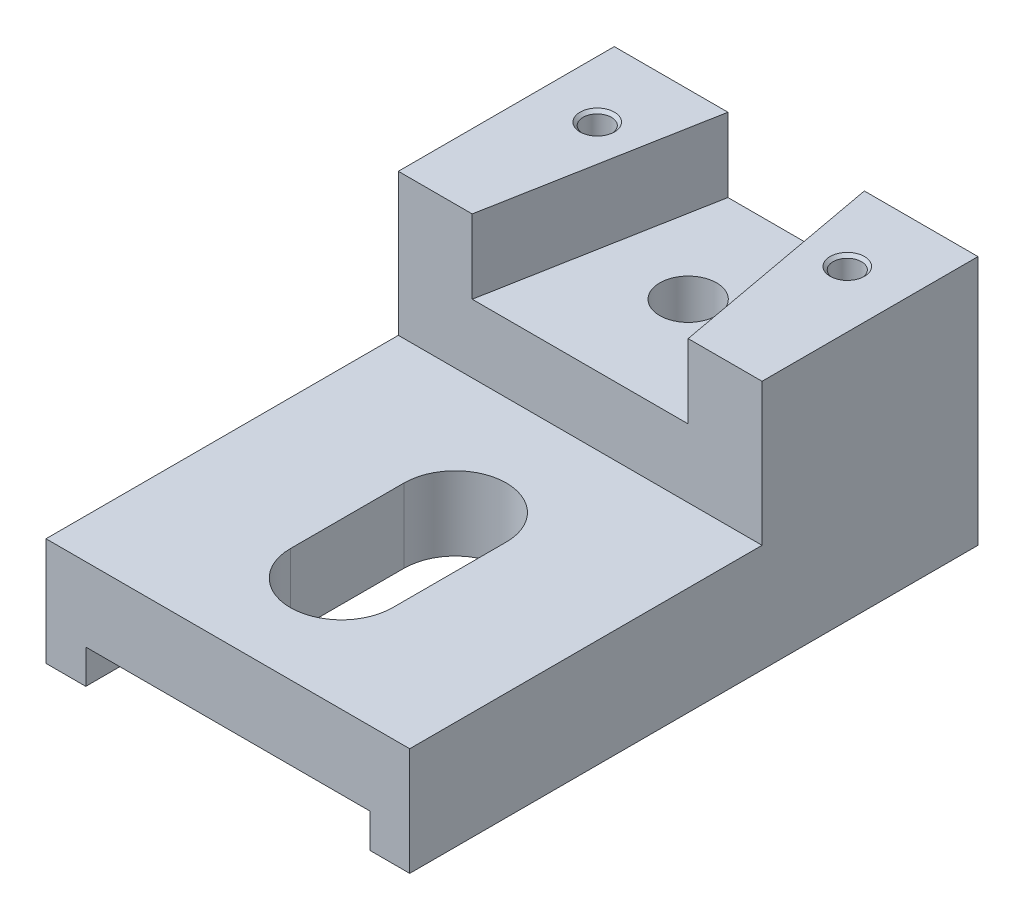
ISO-10303-21;
HEADER;
FILE_DESCRIPTION(('STEP AP214'),'2;1');
FILE_NAME('part.step','',(''),(''),'','','');
FILE_SCHEMA(('AUTOMOTIVE_DESIGN { 1 0 10303 214 1 1 1 1 }'));
ENDSEC;
DATA;
#1=APPLICATION_CONTEXT('core data for automotive mechanical design processes');
#2=APPLICATION_PROTOCOL_DEFINITION('international standard','automotive_design',2000,#1);
#3=PRODUCT_CONTEXT('',#1,'mechanical');
#4=PRODUCT('Part','Part','',(#3));
#5=PRODUCT_RELATED_PRODUCT_CATEGORY('part','',(#4));
#6=PRODUCT_DEFINITION_FORMATION('','',#4);
#7=PRODUCT_DEFINITION_CONTEXT('part definition',#1,'design');
#8=PRODUCT_DEFINITION('design','',#6,#7);
#9=PRODUCT_DEFINITION_SHAPE('','',#8);
#10=(LENGTH_UNIT() NAMED_UNIT(*) SI_UNIT(.MILLI.,.METRE.));
#11=(NAMED_UNIT(*) PLANE_ANGLE_UNIT() SI_UNIT($,.RADIAN.));
#12=(NAMED_UNIT(*) SI_UNIT($,.STERADIAN.) SOLID_ANGLE_UNIT());
#13=UNCERTAINTY_MEASURE_WITH_UNIT(LENGTH_MEASURE(1.E-05),#10,'distance_accuracy_value','');
#14=(GEOMETRIC_REPRESENTATION_CONTEXT(3) GLOBAL_UNCERTAINTY_ASSIGNED_CONTEXT((#13)) GLOBAL_UNIT_ASSIGNED_CONTEXT((#10,
#11,#12)) REPRESENTATION_CONTEXT('',''));
#15=CARTESIAN_POINT('',(0.,0.,0.));
#16=DIRECTION('',(0.,0.,1.));
#17=DIRECTION('',(1.,0.,0.));
#18=AXIS2_PLACEMENT_3D('',#15,#16,#17);
#19=CARTESIAN_POINT('',(-19.,38.,-62.));
#20=DIRECTION('',(-0.983453188589073,0.,-0.181162429476935));
#21=DIRECTION('',(-0.181162429476935,0.,0.983453188589073));
#22=AXIS2_PLACEMENT_3D('',#19,#20,#21);
#23=PLANE('',#22);
#24=DIRECTION('',(-0.181162429476935,0.,0.983453188589073));
#25=VECTOR('',#24,1.);
#26=CARTESIAN_POINT('',(-19.,25.,-62.));
#27=LINE('',#26,#25);
#28=CARTESIAN_POINT('',(-12.,25.,-100.));
#29=VERTEX_POINT('',#28);
#30=CARTESIAN_POINT('',(-19.,25.,-62.));
#31=VERTEX_POINT('',#30);
#32=EDGE_CURVE('E204',#29,#31,#27,.T.);
#33=ORIENTED_EDGE('',*,*,#32,.F.);
#34=DIRECTION('',(0.,-1.,0.));
#35=VECTOR('',#34,1.);
#36=CARTESIAN_POINT('',(-12.,38.,-100.));
#37=LINE('',#36,#35);
#38=CARTESIAN_POINT('',(-12.,38.,-100.));
#39=VERTEX_POINT('',#38);
#40=EDGE_CURVE('E233',#39,#29,#37,.T.);
#41=ORIENTED_EDGE('',*,*,#40,.F.);
#42=DIRECTION('',(0.181162429476935,0.,-0.983453188589073));
#43=VECTOR('',#42,1.);
#44=CARTESIAN_POINT('',(-19.,38.,-62.));
#45=LINE('',#44,#43);
#46=CARTESIAN_POINT('',(-19.,38.,-62.));
#47=VERTEX_POINT('',#46);
#48=EDGE_CURVE('E248',#47,#39,#45,.T.);
#49=ORIENTED_EDGE('',*,*,#48,.F.);
#50=DIRECTION('',(0.,-1.,0.));
#51=VECTOR('',#50,1.);
#52=CARTESIAN_POINT('',(-19.,38.,-62.));
#53=LINE('',#52,#51);
#54=EDGE_CURVE('E261',#47,#31,#53,.T.);
#55=ORIENTED_EDGE('',*,*,#54,.T.);
#56=EDGE_LOOP('',(#33,#41,#49,#55));
#57=FACE_BOUND('',#56,.T.);
#58=ADVANCED_FACE('F43',(#57),#23,.F.);
#59=CARTESIAN_POINT('',(19.,38.,-62.));
#60=DIRECTION('',(0.983453188589073,0.,-0.181162429476935));
#61=DIRECTION('',(-0.181162429476935,0.,-0.983453188589073));
#62=AXIS2_PLACEMENT_3D('',#59,#60,#61);
#63=PLANE('',#62);
#64=DIRECTION('',(-0.181162429476935,0.,-0.983453188589073));
#65=VECTOR('',#64,1.);
#66=CARTESIAN_POINT('',(12.,25.,-100.));
#67=LINE('',#66,#65);
#68=CARTESIAN_POINT('',(19.,25.,-62.));
#69=VERTEX_POINT('',#68);
#70=CARTESIAN_POINT('',(12.,25.,-100.));
#71=VERTEX_POINT('',#70);
#72=EDGE_CURVE('E207',#69,#71,#67,.T.);
#73=ORIENTED_EDGE('',*,*,#72,.F.);
#74=DIRECTION('',(0.,-1.,0.));
#75=VECTOR('',#74,1.);
#76=CARTESIAN_POINT('',(19.,38.,-62.));
#77=LINE('',#76,#75);
#78=CARTESIAN_POINT('',(19.,38.,-62.));
#79=VERTEX_POINT('',#78);
#80=EDGE_CURVE('E249',#79,#69,#77,.T.);
#81=ORIENTED_EDGE('',*,*,#80,.F.);
#82=DIRECTION('',(0.181162429476935,0.,0.983453188589073));
#83=VECTOR('',#82,1.);
#84=CARTESIAN_POINT('',(19.,38.,-62.));
#85=LINE('',#84,#83);
#86=CARTESIAN_POINT('',(12.,38.,-100.));
#87=VERTEX_POINT('',#86);
#88=EDGE_CURVE('E232',#87,#79,#85,.T.);
#89=ORIENTED_EDGE('',*,*,#88,.F.);
#90=DIRECTION('',(0.,-1.,0.));
#91=VECTOR('',#90,1.);
#92=CARTESIAN_POINT('',(12.,38.,-100.));
#93=LINE('',#92,#91);
#94=EDGE_CURVE('E252',#87,#71,#93,.T.);
#95=ORIENTED_EDGE('',*,*,#94,.T.);
#96=EDGE_LOOP('',(#73,#81,#89,#95));
#97=FACE_BOUND('',#96,.T.);
#98=ADVANCED_FACE('F363',(#97),#63,.F.);
#99=CARTESIAN_POINT('',(-25.,0.,-100.));
#100=DIRECTION('',(1.,0.,0.));
#101=DIRECTION('',(0.,0.,-1.));
#102=AXIS2_PLACEMENT_3D('',#99,#100,#101);
#103=PLANE('',#102);
#104=DIRECTION('',(0.,1.,0.));
#105=VECTOR('',#104,1.);
#106=CARTESIAN_POINT('',(-25.,0.,0.));
#107=LINE('',#106,#105);
#108=CARTESIAN_POINT('',(-25.,-6.00000000000001,0.));
#109=VERTEX_POINT('',#108);
#110=CARTESIAN_POINT('',(-25.,0.,0.));
#111=VERTEX_POINT('',#110);
#112=EDGE_CURVE('E254',#109,#111,#107,.T.);
#113=ORIENTED_EDGE('',*,*,#112,.F.);
#114=DIRECTION('',(0.,0.,1.));
#115=VECTOR('',#114,1.);
#116=CARTESIAN_POINT('',(-25.,-6.00000000000001,-100.));
#117=LINE('',#116,#115);
#118=CARTESIAN_POINT('',(-25.,-6.00000000000001,-100.));
#119=VERTEX_POINT('',#118);
#120=EDGE_CURVE('E320',#119,#109,#117,.T.);
#121=ORIENTED_EDGE('',*,*,#120,.F.);
#122=DIRECTION('',(0.,1.,0.));
#123=VECTOR('',#122,1.);
#124=CARTESIAN_POINT('',(-25.,0.,-100.));
#125=LINE('',#124,#123);
#126=CARTESIAN_POINT('',(-25.,0.,-100.));
#127=VERTEX_POINT('',#126);
#128=EDGE_CURVE('E272',#119,#127,#125,.T.);
#129=ORIENTED_EDGE('',*,*,#128,.T.);
#130=DIRECTION('',(0.,0.,1.));
#131=VECTOR('',#130,1.);
#132=CARTESIAN_POINT('',(-25.,0.,-100.));
#133=LINE('',#132,#131);
#134=EDGE_CURVE('E294',#127,#111,#133,.T.);
#135=ORIENTED_EDGE('',*,*,#134,.T.);
#136=EDGE_LOOP('',(#113,#121,#129,#135));
#137=FACE_BOUND('',#136,.T.);
#138=ADVANCED_FACE('F44',(#137),#103,.T.);
#139=CARTESIAN_POINT('',(-25.,-6.00000000000001,-100.));
#140=DIRECTION('',(0.,-1.,0.));
#141=DIRECTION('',(1.,0.,0.));
#142=AXIS2_PLACEMENT_3D('',#139,#140,#141);
#143=PLANE('',#142);
#144=DIRECTION('',(1.,0.,0.));
#145=VECTOR('',#144,1.);
#146=CARTESIAN_POINT('',(-25.,-6.00000000000001,0.));
#147=LINE('',#146,#145);
#148=CARTESIAN_POINT('',(-32.,-6.00000000000001,0.));
#149=VERTEX_POINT('',#148);
#150=EDGE_CURVE('E280',#149,#109,#147,.T.);
#151=ORIENTED_EDGE('',*,*,#150,.F.);
#152=DIRECTION('',(0.,0.,1.));
#153=VECTOR('',#152,1.);
#154=CARTESIAN_POINT('',(-32.,-6.00000000000001,-100.));
#155=LINE('',#154,#153);
#156=CARTESIAN_POINT('',(-32.,-6.00000000000001,-100.));
#157=VERTEX_POINT('',#156);
#158=EDGE_CURVE('E319',#157,#149,#155,.T.);
#159=ORIENTED_EDGE('',*,*,#158,.F.);
#160=DIRECTION('',(1.,0.,0.));
#161=VECTOR('',#160,1.);
#162=CARTESIAN_POINT('',(-25.,-6.00000000000001,-100.));
#163=LINE('',#162,#161);
#164=EDGE_CURVE('E292',#157,#119,#163,.T.);
#165=ORIENTED_EDGE('',*,*,#164,.T.);
#166=ORIENTED_EDGE('',*,*,#120,.T.);
#167=EDGE_LOOP('',(#151,#159,#165,#166));
#168=FACE_BOUND('',#167,.T.);
#169=ADVANCED_FACE('F387',(#168),#143,.T.);
#170=CARTESIAN_POINT('',(-32.,-6.00000000000001,-100.));
#171=DIRECTION('',(-1.,0.,0.));
#172=DIRECTION('',(0.,0.,1.));
#173=AXIS2_PLACEMENT_3D('',#170,#171,#172);
#174=PLANE('',#173);
#175=DIRECTION('',(0.,-1.,0.));
#176=VECTOR('',#175,1.);
#177=CARTESIAN_POINT('',(-32.,-6.00000000000001,0.));
#178=LINE('',#177,#176);
#179=CARTESIAN_POINT('',(-32.,13.,0.));
#180=VERTEX_POINT('',#179);
#181=EDGE_CURVE('E315',#180,#149,#178,.T.);
#182=ORIENTED_EDGE('',*,*,#181,.F.);
#183=DIRECTION('',(0.,0.,1.));
#184=VECTOR('',#183,1.);
#185=CARTESIAN_POINT('',(-32.,13.,-100.));
#186=LINE('',#185,#184);
#187=CARTESIAN_POINT('',(-32.,13.,-62.));
#188=VERTEX_POINT('',#187);
#189=EDGE_CURVE('E325',#188,#180,#186,.T.);
#190=ORIENTED_EDGE('',*,*,#189,.F.);
#191=DIRECTION('',(0.,-1.,0.));
#192=VECTOR('',#191,1.);
#193=CARTESIAN_POINT('',(-32.,38.,-62.));
#194=LINE('',#193,#192);
#195=CARTESIAN_POINT('',(-32.,38.,-62.));
#196=VERTEX_POINT('',#195);
#197=EDGE_CURVE('E256',#196,#188,#194,.T.);
#198=ORIENTED_EDGE('',*,*,#197,.F.);
#199=DIRECTION('',(0.,0.,1.));
#200=VECTOR('',#199,1.);
#201=CARTESIAN_POINT('',(-32.,38.,-100.));
#202=LINE('',#201,#200);
#203=CARTESIAN_POINT('',(-32.,38.,-100.));
#204=VERTEX_POINT('',#203);
#205=EDGE_CURVE('E266',#204,#196,#202,.T.);
#206=ORIENTED_EDGE('',*,*,#205,.F.);
#207=DIRECTION('',(0.,-1.,0.));
#208=VECTOR('',#207,1.);
#209=CARTESIAN_POINT('',(-32.,-6.00000000000001,-100.));
#210=LINE('',#209,#208);
#211=EDGE_CURVE('E286',#204,#157,#210,.T.);
#212=ORIENTED_EDGE('',*,*,#211,.T.);
#213=ORIENTED_EDGE('',*,*,#158,.T.);
#214=EDGE_LOOP('',(#182,#190,#198,#206,#212,#213));
#215=FACE_BOUND('',#214,.T.);
#216=ADVANCED_FACE('F386',(#215),#174,.T.);
#217=CARTESIAN_POINT('',(-32.,13.,-100.));
#218=DIRECTION('',(0.,1.,0.));
#219=DIRECTION('',(-1.,0.,0.));
#220=AXIS2_PLACEMENT_3D('',#217,#218,#219);
#221=PLANE('',#220);
#222=CARTESIAN_POINT('',(0.,13.,-20.));
#223=DIRECTION('',(0.,1.,0.));
#224=DIRECTION('',(-1.,0.,0.));
#225=AXIS2_PLACEMENT_3D('',#222,#223,#224);
#226=CIRCLE('',#225,9.);
#227=CARTESIAN_POINT('',(-9.,13.,-20.));
#228=VERTEX_POINT('',#227);
#229=CARTESIAN_POINT('',(9.,13.,-20.));
#230=VERTEX_POINT('',#229);
#231=EDGE_CURVE('E59',#228,#230,#226,.T.);
#232=ORIENTED_EDGE('',*,*,#231,.F.);
#233=DIRECTION('',(0.,0.,1.));
#234=VECTOR('',#233,1.);
#235=CARTESIAN_POINT('',(-9.,13.,-20.));
#236=LINE('',#235,#234);
#237=CARTESIAN_POINT('',(-9.,13.,-40.));
#238=VERTEX_POINT('',#237);
#239=EDGE_CURVE('E195',#238,#228,#236,.T.);
#240=ORIENTED_EDGE('',*,*,#239,.F.);
#241=CARTESIAN_POINT('',(0.,13.,-40.));
#242=DIRECTION('',(0.,1.,0.));
#243=DIRECTION('',(-1.,0.,0.));
#244=AXIS2_PLACEMENT_3D('',#241,#242,#243);
#245=CIRCLE('',#244,9.);
#246=CARTESIAN_POINT('',(9.,13.,-40.));
#247=VERTEX_POINT('',#246);
#248=EDGE_CURVE('E178',#247,#238,#245,.T.);
#249=ORIENTED_EDGE('',*,*,#248,.F.);
#250=DIRECTION('',(0.,0.,-1.));
#251=VECTOR('',#250,1.);
#252=CARTESIAN_POINT('',(9.,13.,-20.));
#253=LINE('',#252,#251);
#254=EDGE_CURVE('E183',#230,#247,#253,.T.);
#255=ORIENTED_EDGE('',*,*,#254,.F.);
#256=EDGE_LOOP('',(#232,#240,#249,#255));
#257=FACE_BOUND('',#256,.T.);
#258=DIRECTION('',(1.,0.,0.));
#259=VECTOR('',#258,1.);
#260=CARTESIAN_POINT('',(32.,13.,-62.));
#261=LINE('',#260,#259);
#262=CARTESIAN_POINT('',(32.,13.,-62.));
#263=VERTEX_POINT('',#262);
#264=EDGE_CURVE('E237',#188,#263,#261,.T.);
#265=ORIENTED_EDGE('',*,*,#264,.F.);
#266=ORIENTED_EDGE('',*,*,#189,.T.);
#267=DIRECTION('',(-1.,0.,0.));
#268=VECTOR('',#267,1.);
#269=CARTESIAN_POINT('',(-32.,13.,0.));
#270=LINE('',#269,#268);
#271=CARTESIAN_POINT('',(32.,13.,0.));
#272=VERTEX_POINT('',#271);
#273=EDGE_CURVE('E310',#272,#180,#270,.T.);
#274=ORIENTED_EDGE('',*,*,#273,.F.);
#275=DIRECTION('',(0.,0.,1.));
#276=VECTOR('',#275,1.);
#277=CARTESIAN_POINT('',(32.,13.,-100.));
#278=LINE('',#277,#276);
#279=EDGE_CURVE('E322',#263,#272,#278,.T.);
#280=ORIENTED_EDGE('',*,*,#279,.F.);
#281=EDGE_LOOP('',(#265,#266,#274,#280));
#282=FACE_BOUND('',#281,.T.);
#283=ADVANCED_FACE('F187',(#257,#282),#221,.T.);
#284=CARTESIAN_POINT('',(32.,13.,-100.));
#285=DIRECTION('',(1.,0.,0.));
#286=DIRECTION('',(0.,0.,-1.));
#287=AXIS2_PLACEMENT_3D('',#284,#285,#286);
#288=PLANE('',#287);
#289=DIRECTION('',(0.,1.,0.));
#290=VECTOR('',#289,1.);
#291=CARTESIAN_POINT('',(32.,13.,0.));
#292=LINE('',#291,#290);
#293=CARTESIAN_POINT('',(32.,-5.99999999999999,0.));
#294=VERTEX_POINT('',#293);
#295=EDGE_CURVE('E308',#294,#272,#292,.T.);
#296=ORIENTED_EDGE('',*,*,#295,.F.);
#297=DIRECTION('',(0.,0.,1.));
#298=VECTOR('',#297,1.);
#299=CARTESIAN_POINT('',(32.,-5.99999999999999,-100.));
#300=LINE('',#299,#298);
#301=CARTESIAN_POINT('',(32.,-5.99999999999999,-100.));
#302=VERTEX_POINT('',#301);
#303=EDGE_CURVE('E326',#302,#294,#300,.T.);
#304=ORIENTED_EDGE('',*,*,#303,.F.);
#305=DIRECTION('',(0.,1.,0.));
#306=VECTOR('',#305,1.);
#307=CARTESIAN_POINT('',(32.,13.,-100.));
#308=LINE('',#307,#306);
#309=CARTESIAN_POINT('',(32.,38.,-100.));
#310=VERTEX_POINT('',#309);
#311=EDGE_CURVE('E288',#302,#310,#308,.T.);
#312=ORIENTED_EDGE('',*,*,#311,.T.);
#313=DIRECTION('',(0.,0.,-1.));
#314=VECTOR('',#313,1.);
#315=CARTESIAN_POINT('',(32.,38.,-100.));
#316=LINE('',#315,#314);
#317=CARTESIAN_POINT('',(32.,38.,-62.));
#318=VERTEX_POINT('',#317);
#319=EDGE_CURVE('E238',#318,#310,#316,.T.);
#320=ORIENTED_EDGE('',*,*,#319,.F.);
#321=DIRECTION('',(0.,-1.,0.));
#322=VECTOR('',#321,1.);
#323=CARTESIAN_POINT('',(32.,38.,-62.));
#324=LINE('',#323,#322);
#325=EDGE_CURVE('E241',#318,#263,#324,.T.);
#326=ORIENTED_EDGE('',*,*,#325,.T.);
#327=ORIENTED_EDGE('',*,*,#279,.T.);
#328=EDGE_LOOP('',(#296,#304,#312,#320,#326,#327));
#329=FACE_BOUND('',#328,.T.);
#330=ADVANCED_FACE('F394',(#329),#288,.T.);
#331=CARTESIAN_POINT('',(32.,-5.99999999999999,-100.));
#332=DIRECTION('',(0.,-1.,0.));
#333=DIRECTION('',(1.,0.,0.));
#334=AXIS2_PLACEMENT_3D('',#331,#332,#333);
#335=PLANE('',#334);
#336=DIRECTION('',(1.,0.,0.));
#337=VECTOR('',#336,1.);
#338=CARTESIAN_POINT('',(32.,-5.99999999999999,0.));
#339=LINE('',#338,#337);
#340=CARTESIAN_POINT('',(25.,-5.99999999999999,0.));
#341=VERTEX_POINT('',#340);
#342=EDGE_CURVE('E301',#341,#294,#339,.T.);
#343=ORIENTED_EDGE('',*,*,#342,.F.);
#344=DIRECTION('',(0.,0.,1.));
#345=VECTOR('',#344,1.);
#346=CARTESIAN_POINT('',(25.,-5.99999999999999,-100.));
#347=LINE('',#346,#345);
#348=CARTESIAN_POINT('',(25.,-5.99999999999999,-100.));
#349=VERTEX_POINT('',#348);
#350=EDGE_CURVE('E327',#349,#341,#347,.T.);
#351=ORIENTED_EDGE('',*,*,#350,.F.);
#352=DIRECTION('',(1.,0.,0.));
#353=VECTOR('',#352,1.);
#354=CARTESIAN_POINT('',(32.,-5.99999999999999,-100.));
#355=LINE('',#354,#353);
#356=EDGE_CURVE('E281',#349,#302,#355,.T.);
#357=ORIENTED_EDGE('',*,*,#356,.T.);
#358=ORIENTED_EDGE('',*,*,#303,.T.);
#359=EDGE_LOOP('',(#343,#351,#357,#358));
#360=FACE_BOUND('',#359,.T.);
#361=ADVANCED_FACE('F396',(#360),#335,.T.);
#362=CARTESIAN_POINT('',(25.,-5.99999999999999,-100.));
#363=DIRECTION('',(-1.,0.,0.));
#364=DIRECTION('',(0.,0.,1.));
#365=AXIS2_PLACEMENT_3D('',#362,#363,#364);
#366=PLANE('',#365);
#367=DIRECTION('',(0.,-1.,0.));
#368=VECTOR('',#367,1.);
#369=CARTESIAN_POINT('',(25.,-5.99999999999999,0.));
#370=LINE('',#369,#368);
#371=CARTESIAN_POINT('',(25.,0.,0.));
#372=VERTEX_POINT('',#371);
#373=EDGE_CURVE('E299',#372,#341,#370,.T.);
#374=ORIENTED_EDGE('',*,*,#373,.F.);
#375=DIRECTION('',(0.,0.,1.));
#376=VECTOR('',#375,1.);
#377=CARTESIAN_POINT('',(25.,0.,-100.));
#378=LINE('',#377,#376);
#379=CARTESIAN_POINT('',(25.,0.,-100.));
#380=VERTEX_POINT('',#379);
#381=EDGE_CURVE('E329',#380,#372,#378,.T.);
#382=ORIENTED_EDGE('',*,*,#381,.F.);
#383=DIRECTION('',(0.,-1.,0.));
#384=VECTOR('',#383,1.);
#385=CARTESIAN_POINT('',(25.,-5.99999999999999,-100.));
#386=LINE('',#385,#384);
#387=EDGE_CURVE('E278',#380,#349,#386,.T.);
#388=ORIENTED_EDGE('',*,*,#387,.T.);
#389=ORIENTED_EDGE('',*,*,#350,.T.);
#390=EDGE_LOOP('',(#374,#382,#388,#389));
#391=FACE_BOUND('',#390,.T.);
#392=ADVANCED_FACE('F405',(#391),#366,.T.);
#393=CARTESIAN_POINT('',(25.,0.,-100.));
#394=DIRECTION('',(0.,-1.,0.));
#395=DIRECTION('',(0.,0.,-1.));
#396=AXIS2_PLACEMENT_3D('',#393,#394,#395);
#397=PLANE('',#396);
#398=CARTESIAN_POINT('',(0.,0.,-20.));
#399=DIRECTION('',(0.,-1.,0.));
#400=DIRECTION('',(0.,0.,-1.));
#401=AXIS2_PLACEMENT_3D('',#398,#399,#400);
#402=CIRCLE('',#401,9.);
#403=CARTESIAN_POINT('',(9.,0.,-20.));
#404=VERTEX_POINT('',#403);
#405=CARTESIAN_POINT('',(-9.,0.,-20.));
#406=VERTEX_POINT('',#405);
#407=EDGE_CURVE('E11',#404,#406,#402,.T.);
#408=ORIENTED_EDGE('',*,*,#407,.F.);
#409=DIRECTION('',(0.,0.,1.));
#410=VECTOR('',#409,1.);
#411=CARTESIAN_POINT('',(9.,0.,-100.));
#412=LINE('',#411,#410);
#413=CARTESIAN_POINT('',(9.,0.,-40.));
#414=VERTEX_POINT('',#413);
#415=EDGE_CURVE('E333',#414,#404,#412,.T.);
#416=ORIENTED_EDGE('',*,*,#415,.F.);
#417=CARTESIAN_POINT('',(0.,0.,-40.));
#418=DIRECTION('',(0.,-1.,0.));
#419=DIRECTION('',(0.,0.,-1.));
#420=AXIS2_PLACEMENT_3D('',#417,#418,#419);
#421=CIRCLE('',#420,9.);
#422=CARTESIAN_POINT('',(-9.,0.,-40.));
#423=VERTEX_POINT('',#422);
#424=EDGE_CURVE('E179',#423,#414,#421,.T.);
#425=ORIENTED_EDGE('',*,*,#424,.F.);
#426=DIRECTION('',(0.,0.,-1.));
#427=VECTOR('',#426,1.);
#428=CARTESIAN_POINT('',(-8.99999999999999,0.,-100.));
#429=LINE('',#428,#427);
#430=EDGE_CURVE('E51',#406,#423,#429,.T.);
#431=ORIENTED_EDGE('',*,*,#430,.F.);
#432=EDGE_LOOP('',(#408,#416,#425,#431));
#433=FACE_BOUND('',#432,.T.);
#434=DIRECTION('',(1.,0.,0.));
#435=VECTOR('',#434,1.);
#436=CARTESIAN_POINT('',(25.,0.,0.));
#437=LINE('',#436,#435);
#438=EDGE_CURVE('E300',#111,#372,#437,.T.);
#439=ORIENTED_EDGE('',*,*,#438,.F.);
#440=ORIENTED_EDGE('',*,*,#134,.F.);
#441=DIRECTION('',(1.,0.,0.));
#442=VECTOR('',#441,1.);
#443=CARTESIAN_POINT('',(25.,0.,-100.));
#444=LINE('',#443,#442);
#445=EDGE_CURVE('E277',#127,#380,#444,.T.);
#446=ORIENTED_EDGE('',*,*,#445,.T.);
#447=ORIENTED_EDGE('',*,*,#381,.T.);
#448=EDGE_LOOP('',(#439,#440,#446,#447));
#449=FACE_BOUND('',#448,.T.);
#450=ADVANCED_FACE('F341',(#433,#449),#397,.T.);
#451=CARTESIAN_POINT('',(0.,0.,-100.));
#452=DIRECTION('',(0.,0.,-1.));
#453=DIRECTION('',(-1.,0.,0.));
#454=AXIS2_PLACEMENT_3D('',#451,#452,#453);
#455=PLANE('',#454);
#456=ORIENTED_EDGE('',*,*,#128,.F.);
#457=ORIENTED_EDGE('',*,*,#164,.F.);
#458=ORIENTED_EDGE('',*,*,#211,.F.);
#459=DIRECTION('',(-1.,0.,0.));
#460=VECTOR('',#459,1.);
#461=CARTESIAN_POINT('',(-12.,38.,-100.));
#462=LINE('',#461,#460);
#463=EDGE_CURVE('E268',#39,#204,#462,.T.);
#464=ORIENTED_EDGE('',*,*,#463,.F.);
#465=ORIENTED_EDGE('',*,*,#40,.T.);
#466=DIRECTION('',(-1.,0.,0.));
#467=VECTOR('',#466,1.);
#468=CARTESIAN_POINT('',(-12.,25.,-100.));
#469=LINE('',#468,#467);
#470=EDGE_CURVE('E211',#71,#29,#469,.T.);
#471=ORIENTED_EDGE('',*,*,#470,.F.);
#472=ORIENTED_EDGE('',*,*,#94,.F.);
#473=DIRECTION('',(-1.,0.,0.));
#474=VECTOR('',#473,1.);
#475=CARTESIAN_POINT('',(12.,38.,-100.));
#476=LINE('',#475,#474);
#477=EDGE_CURVE('E235',#310,#87,#476,.T.);
#478=ORIENTED_EDGE('',*,*,#477,.F.);
#479=ORIENTED_EDGE('',*,*,#311,.F.);
#480=ORIENTED_EDGE('',*,*,#356,.F.);
#481=ORIENTED_EDGE('',*,*,#387,.F.);
#482=ORIENTED_EDGE('',*,*,#445,.F.);
#483=EDGE_LOOP('',(#456,#457,#458,#464,#465,#471,#472,#478,#479,#480,#481,#482));
#484=FACE_BOUND('',#483,.T.);
#485=ADVANCED_FACE('F377',(#484),#455,.T.);
#486=CARTESIAN_POINT('',(0.,0.,0.));
#487=DIRECTION('',(0.,0.,-1.));
#488=DIRECTION('',(-1.,0.,0.));
#489=AXIS2_PLACEMENT_3D('',#486,#487,#488);
#490=PLANE('',#489);
#491=ORIENTED_EDGE('',*,*,#112,.T.);
#492=ORIENTED_EDGE('',*,*,#438,.T.);
#493=ORIENTED_EDGE('',*,*,#373,.T.);
#494=ORIENTED_EDGE('',*,*,#342,.T.);
#495=ORIENTED_EDGE('',*,*,#295,.T.);
#496=ORIENTED_EDGE('',*,*,#273,.T.);
#497=ORIENTED_EDGE('',*,*,#181,.T.);
#498=ORIENTED_EDGE('',*,*,#150,.T.);
#499=EDGE_LOOP('',(#491,#492,#493,#494,#495,#496,#497,#498));
#500=FACE_BOUND('',#499,.T.);
#501=ADVANCED_FACE('F380',(#500),#490,.F.);
#502=CARTESIAN_POINT('',(0.,38.,0.));
#503=DIRECTION('',(0.,1.,0.));
#504=DIRECTION('',(-1.,0.,0.));
#505=AXIS2_PLACEMENT_3D('',#502,#503,#504);
#506=PLANE('',#505);
#507=CARTESIAN_POINT('',(-22.,38.,-87.));
#508=DIRECTION('',(0.,1.,0.));
#509=DIRECTION('',(0.,0.,1.));
#510=AXIS2_PLACEMENT_3D('',#507,#508,#509);
#511=CIRCLE('',#510,3.025);
#512=CARTESIAN_POINT('',(-22.,38.,-83.975));
#513=VERTEX_POINT('',#512);
#514=EDGE_CURVE('E225',#513,#513,#511,.T.);
#515=ORIENTED_EDGE('',*,*,#514,.F.);
#516=EDGE_LOOP('',(#515));
#517=FACE_BOUND('',#516,.T.);
#518=ORIENTED_EDGE('',*,*,#48,.T.);
#519=ORIENTED_EDGE('',*,*,#463,.T.);
#520=ORIENTED_EDGE('',*,*,#205,.T.);
#521=DIRECTION('',(1.,0.,0.));
#522=VECTOR('',#521,1.);
#523=CARTESIAN_POINT('',(-32.,38.,-62.));
#524=LINE('',#523,#522);
#525=EDGE_CURVE('E262',#196,#47,#524,.T.);
#526=ORIENTED_EDGE('',*,*,#525,.T.);
#527=EDGE_LOOP('',(#518,#519,#520,#526));
#528=FACE_BOUND('',#527,.T.);
#529=ADVANCED_FACE('F373',(#517,#528),#506,.T.);
#530=CARTESIAN_POINT('',(32.,38.,-62.));
#531=DIRECTION('',(0.,0.,-1.));
#532=DIRECTION('',(-1.,0.,0.));
#533=AXIS2_PLACEMENT_3D('',#530,#531,#532);
#534=PLANE('',#533);
#535=ORIENTED_EDGE('',*,*,#264,.T.);
#536=ORIENTED_EDGE('',*,*,#325,.F.);
#537=DIRECTION('',(1.,0.,0.));
#538=VECTOR('',#537,1.);
#539=CARTESIAN_POINT('',(32.,38.,-62.));
#540=LINE('',#539,#538);
#541=EDGE_CURVE('E236',#79,#318,#540,.T.);
#542=ORIENTED_EDGE('',*,*,#541,.F.);
#543=ORIENTED_EDGE('',*,*,#80,.T.);
#544=DIRECTION('',(1.,0.,0.));
#545=VECTOR('',#544,1.);
#546=CARTESIAN_POINT('',(19.,25.,-62.));
#547=LINE('',#546,#545);
#548=EDGE_CURVE('E210',#31,#69,#547,.T.);
#549=ORIENTED_EDGE('',*,*,#548,.F.);
#550=ORIENTED_EDGE('',*,*,#54,.F.);
#551=ORIENTED_EDGE('',*,*,#525,.F.);
#552=ORIENTED_EDGE('',*,*,#197,.T.);
#553=EDGE_LOOP('',(#535,#536,#542,#543,#549,#550,#551,#552));
#554=FACE_BOUND('',#553,.T.);
#555=ADVANCED_FACE('F376',(#554),#534,.F.);
#556=CARTESIAN_POINT('',(0.,38.,0.));
#557=DIRECTION('',(0.,-1.,0.));
#558=DIRECTION('',(1.,0.,0.));
#559=AXIS2_PLACEMENT_3D('',#556,#557,#558);
#560=PLANE('',#559);
#561=CARTESIAN_POINT('',(22.,38.,-87.));
#562=DIRECTION('',(0.,1.,0.));
#563=DIRECTION('',(0.,0.,1.));
#564=AXIS2_PLACEMENT_3D('',#561,#562,#563);
#565=CIRCLE('',#564,3.025);
#566=CARTESIAN_POINT('',(22.,38.,-83.975));
#567=VERTEX_POINT('',#566);
#568=EDGE_CURVE('E213',#567,#567,#565,.T.);
#569=ORIENTED_EDGE('',*,*,#568,.F.);
#570=EDGE_LOOP('',(#569));
#571=FACE_BOUND('',#570,.T.);
#572=ORIENTED_EDGE('',*,*,#477,.T.);
#573=ORIENTED_EDGE('',*,*,#88,.T.);
#574=ORIENTED_EDGE('',*,*,#541,.T.);
#575=ORIENTED_EDGE('',*,*,#319,.T.);
#576=EDGE_LOOP('',(#572,#573,#574,#575));
#577=FACE_BOUND('',#576,.T.);
#578=ADVANCED_FACE('F441',(#571,#577),#560,.F.);
#579=CARTESIAN_POINT('',(-22.,19.5021515475689,-87.));
#580=DIRECTION('',(0.,1.,0.));
#581=DIRECTION('',(0.,0.,1.));
#582=AXIS2_PLACEMENT_3D('',#579,#580,#581);
#583=CONICAL_SURFACE('',#582,2.5,1.02974425867665);
#584=CARTESIAN_POINT('',(-22.,18.,-87.));
#585=VERTEX_POINT('',#584);
#586=VERTEX_LOOP('',#585);
#587=FACE_BOUND('',#586,.T.);
#588=CARTESIAN_POINT('',(-22.,19.5021515475689,-87.));
#589=DIRECTION('',(0.,1.,0.));
#590=DIRECTION('',(0.,0.,1.));
#591=AXIS2_PLACEMENT_3D('',#588,#589,#590);
#592=CIRCLE('',#591,2.5);
#593=CARTESIAN_POINT('',(-22.,19.5021515475689,-84.5));
#594=VERTEX_POINT('',#593);
#595=EDGE_CURVE('E226',#594,#594,#592,.T.);
#596=ORIENTED_EDGE('',*,*,#595,.T.);
#597=EDGE_LOOP('',(#596));
#598=FACE_BOUND('',#597,.T.);
#599=ADVANCED_FACE('F488',(#587,#598),#583,.F.);
#600=CARTESIAN_POINT('',(-22.,38.,-87.));
#601=DIRECTION('',(0.,1.,0.));
#602=DIRECTION('',(0.,0.,1.));
#603=AXIS2_PLACEMENT_3D('',#600,#601,#602);
#604=CYLINDRICAL_SURFACE('',#603,2.5);
#605=ORIENTED_EDGE('',*,*,#595,.F.);
#606=EDGE_LOOP('',(#605));
#607=FACE_BOUND('',#606,.T.);
#608=CARTESIAN_POINT('',(-22.,37.475,-87.));
#609=DIRECTION('',(0.,1.,0.));
#610=DIRECTION('',(0.,0.,1.));
#611=AXIS2_PLACEMENT_3D('',#608,#609,#610);
#612=CIRCLE('',#611,2.5);
#613=CARTESIAN_POINT('',(-22.,37.475,-84.5));
#614=VERTEX_POINT('',#613);
#615=EDGE_CURVE('E223',#614,#614,#612,.T.);
#616=ORIENTED_EDGE('',*,*,#615,.T.);
#617=EDGE_LOOP('',(#616));
#618=FACE_BOUND('',#617,.T.);
#619=ADVANCED_FACE('F496',(#607,#618),#604,.F.);
#620=CARTESIAN_POINT('',(-22.,38.,-87.));
#621=DIRECTION('',(0.,1.,0.));
#622=DIRECTION('',(0.,0.,1.));
#623=AXIS2_PLACEMENT_3D('',#620,#621,#622);
#624=CONICAL_SURFACE('',#623,3.025,0.785398163397445);
#625=ORIENTED_EDGE('',*,*,#615,.F.);
#626=EDGE_LOOP('',(#625));
#627=FACE_BOUND('',#626,.T.);
#628=ORIENTED_EDGE('',*,*,#514,.T.);
#629=EDGE_LOOP('',(#628));
#630=FACE_BOUND('',#629,.T.);
#631=ADVANCED_FACE('F507',(#627,#630),#624,.F.);
#632=CARTESIAN_POINT('',(22.,19.5021515475689,-87.));
#633=DIRECTION('',(0.,1.,0.));
#634=DIRECTION('',(0.,0.,1.));
#635=AXIS2_PLACEMENT_3D('',#632,#633,#634);
#636=CONICAL_SURFACE('',#635,2.5,1.02974425867665);
#637=CARTESIAN_POINT('',(22.,18.,-87.));
#638=VERTEX_POINT('',#637);
#639=VERTEX_LOOP('',#638);
#640=FACE_BOUND('',#639,.T.);
#641=CARTESIAN_POINT('',(22.,19.5021515475689,-87.));
#642=DIRECTION('',(0.,1.,0.));
#643=DIRECTION('',(0.,0.,1.));
#644=AXIS2_PLACEMENT_3D('',#641,#642,#643);
#645=CIRCLE('',#644,2.5);
#646=CARTESIAN_POINT('',(22.,19.5021515475689,-84.5));
#647=VERTEX_POINT('',#646);
#648=EDGE_CURVE('E218',#647,#647,#645,.T.);
#649=ORIENTED_EDGE('',*,*,#648,.T.);
#650=EDGE_LOOP('',(#649));
#651=FACE_BOUND('',#650,.T.);
#652=ADVANCED_FACE('F525',(#640,#651),#636,.F.);
#653=CARTESIAN_POINT('',(22.,38.,-87.));
#654=DIRECTION('',(0.,1.,0.));
#655=DIRECTION('',(0.,0.,1.));
#656=AXIS2_PLACEMENT_3D('',#653,#654,#655);
#657=CYLINDRICAL_SURFACE('',#656,2.5);
#658=ORIENTED_EDGE('',*,*,#648,.F.);
#659=EDGE_LOOP('',(#658));
#660=FACE_BOUND('',#659,.T.);
#661=CARTESIAN_POINT('',(22.,37.475,-87.));
#662=DIRECTION('',(0.,1.,0.));
#663=DIRECTION('',(0.,0.,1.));
#664=AXIS2_PLACEMENT_3D('',#661,#662,#663);
#665=CIRCLE('',#664,2.5);
#666=CARTESIAN_POINT('',(22.,37.475,-84.5));
#667=VERTEX_POINT('',#666);
#668=EDGE_CURVE('E216',#667,#667,#665,.T.);
#669=ORIENTED_EDGE('',*,*,#668,.T.);
#670=EDGE_LOOP('',(#669));
#671=FACE_BOUND('',#670,.T.);
#672=ADVANCED_FACE('F535',(#660,#671),#657,.F.);
#673=CARTESIAN_POINT('',(22.,38.,-87.));
#674=DIRECTION('',(0.,1.,0.));
#675=DIRECTION('',(0.,0.,1.));
#676=AXIS2_PLACEMENT_3D('',#673,#674,#675);
#677=CONICAL_SURFACE('',#676,3.025,0.785398163397445);
#678=ORIENTED_EDGE('',*,*,#668,.F.);
#679=EDGE_LOOP('',(#678));
#680=FACE_BOUND('',#679,.T.);
#681=ORIENTED_EDGE('',*,*,#568,.T.);
#682=EDGE_LOOP('',(#681));
#683=FACE_BOUND('',#682,.T.);
#684=ADVANCED_FACE('F440',(#680,#683),#677,.F.);
#685=CARTESIAN_POINT('',(0.,25.,0.));
#686=DIRECTION('',(0.,-1.,0.));
#687=DIRECTION('',(0.,0.,-1.));
#688=AXIS2_PLACEMENT_3D('',#685,#686,#687);
#689=PLANE('',#688);
#690=ORIENTED_EDGE('',*,*,#32,.T.);
#691=ORIENTED_EDGE('',*,*,#548,.T.);
#692=ORIENTED_EDGE('',*,*,#72,.T.);
#693=ORIENTED_EDGE('',*,*,#470,.T.);
#694=EDGE_LOOP('',(#690,#691,#692,#693));
#695=FACE_BOUND('',#694,.T.);
#696=CARTESIAN_POINT('',(0.,25.,-81.));
#697=DIRECTION('',(0.,1.,0.));
#698=DIRECTION('',(-1.,0.,0.));
#699=AXIS2_PLACEMENT_3D('',#696,#697,#698);
#700=CIRCLE('',#699,5.);
#701=CARTESIAN_POINT('',(-5.00000000000001,25.,-81.));
#702=VERTEX_POINT('',#701);
#703=EDGE_CURVE('E200',#702,#702,#700,.T.);
#704=ORIENTED_EDGE('',*,*,#703,.F.);
#705=EDGE_LOOP('',(#704));
#706=FACE_BOUND('',#705,.T.);
#707=ADVANCED_FACE('F427',(#695,#706),#689,.F.);
#708=CARTESIAN_POINT('',(0.,25.,-81.));
#709=DIRECTION('',(0.,-1.,0.));
#710=DIRECTION('',(1.,0.,0.));
#711=AXIS2_PLACEMENT_3D('',#708,#709,#710);
#712=CYLINDRICAL_SURFACE('',#711,5.);
#713=ORIENTED_EDGE('',*,*,#703,.T.);
#714=EDGE_LOOP('',(#713));
#715=FACE_BOUND('',#714,.T.);
#716=CARTESIAN_POINT('',(0.,13.,-81.));
#717=DIRECTION('',(0.,1.,0.));
#718=DIRECTION('',(-1.,0.,0.));
#719=AXIS2_PLACEMENT_3D('',#716,#717,#718);
#720=CIRCLE('',#719,5.);
#721=CARTESIAN_POINT('',(-5.00000000000001,13.,-81.));
#722=VERTEX_POINT('',#721);
#723=EDGE_CURVE('E317',#722,#722,#720,.F.);
#724=ORIENTED_EDGE('',*,*,#723,.T.);
#725=EDGE_LOOP('',(#724));
#726=FACE_BOUND('',#725,.T.);
#727=ADVANCED_FACE('F354',(#715,#726),#712,.F.);
#728=ORIENTED_EDGE('',*,*,#723,.F.);
#729=EDGE_LOOP('',(#728));
#730=FACE_BOUND('',#729,.T.);
#731=ADVANCED_FACE('F350',(#730),#221,.T.);
#732=CARTESIAN_POINT('',(0.,-6.00000000000001,-20.));
#733=DIRECTION('',(0.,1.,0.));
#734=DIRECTION('',(-1.,0.,0.));
#735=AXIS2_PLACEMENT_3D('',#732,#733,#734);
#736=CYLINDRICAL_SURFACE('',#735,9.);
#737=ORIENTED_EDGE('',*,*,#407,.T.);
#738=DIRECTION('',(0.,1.,0.));
#739=VECTOR('',#738,1.);
#740=CARTESIAN_POINT('',(-9.,-6.00000000000001,-20.));
#741=LINE('',#740,#739);
#742=EDGE_CURVE('E197',#406,#228,#741,.T.);
#743=ORIENTED_EDGE('',*,*,#742,.T.);
#744=ORIENTED_EDGE('',*,*,#231,.T.);
#745=DIRECTION('',(0.,1.,0.));
#746=VECTOR('',#745,1.);
#747=CARTESIAN_POINT('',(9.,-6.00000000000001,-20.));
#748=LINE('',#747,#746);
#749=EDGE_CURVE('E185',#404,#230,#748,.T.);
#750=ORIENTED_EDGE('',*,*,#749,.F.);
#751=EDGE_LOOP('',(#737,#743,#744,#750));
#752=FACE_BOUND('',#751,.T.);
#753=ADVANCED_FACE('F342',(#752),#736,.F.);
#754=CARTESIAN_POINT('',(-9.,-6.00000000000001,-20.));
#755=DIRECTION('',(-1.,0.,0.));
#756=DIRECTION('',(0.,-1.,0.));
#757=AXIS2_PLACEMENT_3D('',#754,#755,#756);
#758=PLANE('',#757);
#759=ORIENTED_EDGE('',*,*,#430,.T.);
#760=DIRECTION('',(0.,1.,0.));
#761=VECTOR('',#760,1.);
#762=CARTESIAN_POINT('',(-9.,-6.00000000000001,-40.));
#763=LINE('',#762,#761);
#764=EDGE_CURVE('E182',#423,#238,#763,.T.);
#765=ORIENTED_EDGE('',*,*,#764,.T.);
#766=ORIENTED_EDGE('',*,*,#239,.T.);
#767=ORIENTED_EDGE('',*,*,#742,.F.);
#768=EDGE_LOOP('',(#759,#765,#766,#767));
#769=FACE_BOUND('',#768,.T.);
#770=ADVANCED_FACE('F339',(#769),#758,.F.);
#771=CARTESIAN_POINT('',(0.,-6.00000000000001,-40.));
#772=DIRECTION('',(0.,1.,0.));
#773=DIRECTION('',(-1.,0.,0.));
#774=AXIS2_PLACEMENT_3D('',#771,#772,#773);
#775=CYLINDRICAL_SURFACE('',#774,9.);
#776=ORIENTED_EDGE('',*,*,#424,.T.);
#777=DIRECTION('',(0.,1.,0.));
#778=VECTOR('',#777,1.);
#779=CARTESIAN_POINT('',(9.,-6.00000000000001,-40.));
#780=LINE('',#779,#778);
#781=EDGE_CURVE('E68',#414,#247,#780,.T.);
#782=ORIENTED_EDGE('',*,*,#781,.T.);
#783=ORIENTED_EDGE('',*,*,#248,.T.);
#784=ORIENTED_EDGE('',*,*,#764,.F.);
#785=EDGE_LOOP('',(#776,#782,#783,#784));
#786=FACE_BOUND('',#785,.T.);
#787=ADVANCED_FACE('F171',(#786),#775,.F.);
#788=CARTESIAN_POINT('',(9.,-6.00000000000001,-20.));
#789=DIRECTION('',(1.,0.,0.));
#790=DIRECTION('',(0.,1.,0.));
#791=AXIS2_PLACEMENT_3D('',#788,#789,#790);
#792=PLANE('',#791);
#793=ORIENTED_EDGE('',*,*,#415,.T.);
#794=ORIENTED_EDGE('',*,*,#749,.T.);
#795=ORIENTED_EDGE('',*,*,#254,.T.);
#796=ORIENTED_EDGE('',*,*,#781,.F.);
#797=EDGE_LOOP('',(#793,#794,#795,#796));
#798=FACE_BOUND('',#797,.T.);
#799=ADVANCED_FACE('F188',(#798),#792,.F.);
#800=CLOSED_SHELL('',(#58,#98,#138,#169,#216,#283,#330,#361,#392,#450,#485,#501,#529,#555,#578,
#599,#619,#631,#652,#672,#684,#707,#727,#731,#753,#770,#787,#799));
#801=MANIFOLD_SOLID_BREP('B2',#800);
#802=ADVANCED_BREP_SHAPE_REPRESENTATION('',(#18,#801),#14);
#803=SHAPE_DEFINITION_REPRESENTATION(#9,#802);
ENDSEC;
END-ISO-10303-21;
